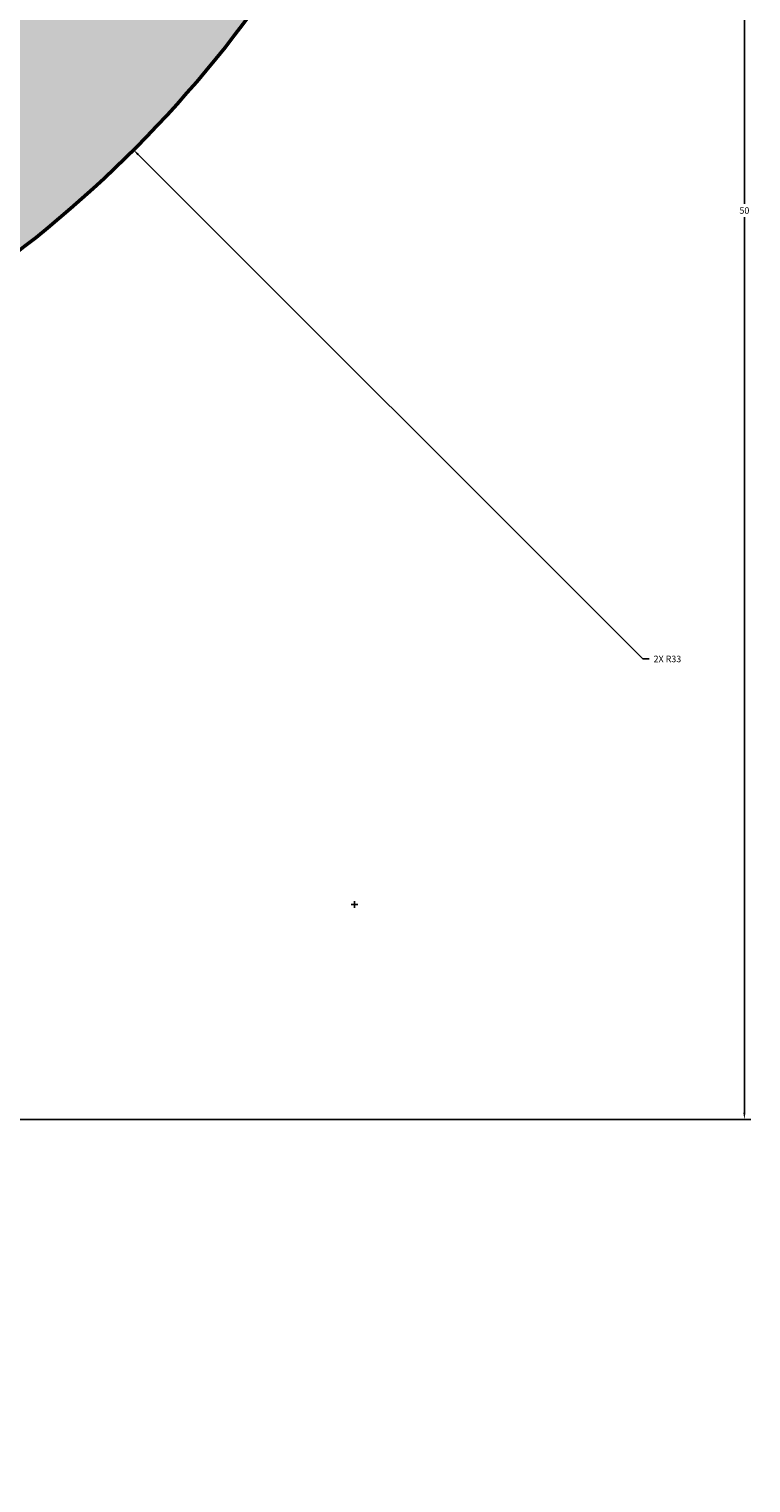
# Model space of a CAD drawing. Units: inches. Extents: x -13 to 107, y -48 to 102.
# Tile 4 of 13: x 48 to 68, y -47 to -7. Entities that reach past the tile are written whole.
import ezdxf

# ---------------------------------------------------------------- set-up
doc = ezdxf.new("R2010")
doc.units = ezdxf.units.IN
doc.header["$MEASUREMENT"] = 0
for name, color, linetype, lineweight in [('M-DIMS', 2, 'Continuous', 18), ('M-HATC', 8, 'Continuous', 18), ('M-OUTL', 7, 'Continuous', 50)]:
    doc.layers.add(name, color=color, linetype=linetype, lineweight=lineweight)
doc.styles.get("Standard").update_dxf_attribs({"font": 'arial.ttf'})
doc.dimstyles.get("Standard").update_dxf_attribs({"dimtxt": 0.18, "dimasz": 0.18, "dimexe": 0.18, "dimexo": 0.0625, "dimgap": 0.09, "dimtad": 0, "dimtih": 1, "dimtoh": 1, "dimdec": 4, "dimzin": 0, "dimdsep": 46, "dimtxsty": 'Standard', "dimcen": 0.09, "dimadec": 0, "dimazin": 0, "dimtfac": 1, "dimtdec": 4, "dimtofl": 0, "dimtmove": 0, "dimatfit": 3, "dimfxl": 1, "dimtolj": 1, "dimtzin": 0, "dimarcsym": 0})

# ---------------------------------------------------------------- blocks, each defined once
blk = doc.blocks.new('*D3')
at = {"layer": 'Defpoints', "color": 0, "transparency": 16777216}
for p in [(27.547, 13.408), (67.679, 13.408), (27.547, -36.592)]:
    blk.add_point(p, dxfattribs=at)
at = {"layer": 'M-DIMS', "color": 0, "lineweight": -2, "transparency": 16777216}
for p, q in [((27.609, 13.408), (67.859, 13.408)), ((67.679, 13.228), (67.679, -11.41)), ((67.679, -36.412), (67.679, -11.774)), ((27.609, -36.592), (67.859, -36.592))]:
    blk.add_line(p, q, dxfattribs=at)
at = {"layer": 'M-DIMS', "color": 0, "transparency": 16777216}
for points in [[(67.649, 13.228), (67.709, 13.228), (67.679, 13.408)], [(67.649, -36.412), (67.709, -36.412), (67.679, -36.592)]]:
    blk.add_solid(points, dxfattribs=at)
at = {"layer": 'M-DIMS', "color": 0, "transparency": 16777216, "insert": (67.679, -11.592), "char_height": 0.18, "attachment_point": 5}
blk.add_mtext('\\A1;50', dxfattribs=at)
blk = doc.blocks.new('*D8')
at = {"layer": 'Defpoints', "color": 0, "transparency": 16777216}
for p in [(27.547, 13.408), (50.882, -9.927)]:
    blk.add_point(p, dxfattribs=at)
at = {"layer": 'M-DIMS', "color": 0, "lineweight": -2, "transparency": 16777216}
for p, q in [((27.457, 13.408), (27.637, 13.408)), ((27.547, 13.318), (27.547, 13.498)), ((64.882, -23.927), (51.009, -10.054)), ((65.062, -23.927), (64.882, -23.927))]:
    blk.add_line(p, q, dxfattribs=at)
at = {"layer": 'M-DIMS', "color": 0, "transparency": 16777216}
blk.add_solid([(51.03, -10.033), (50.988, -10.075), (50.882, -9.927)], dxfattribs=at)
at = {"layer": 'M-DIMS', "color": 0, "transparency": 16777216, "insert": (65.562, -23.927), "char_height": 0.18, "attachment_point": 5}
blk.add_mtext('\\A1;2X R33', dxfattribs=at)
blk = doc.blocks.new('*D11')
at = {"layer": 'Defpoints', "color": 0, "transparency": 16777216}
for p in [(38.592, -22.767), (56.959, -30.682)]:
    blk.add_point(p, dxfattribs=at)
at = {"layer": 'M-DIMS', "color": 0, "lineweight": -2, "transparency": 16777216}
for p, q in [((27.392, -18.018), (27.572, -18.018)), ((27.572, -18.018), (38.427, -22.696)), ((56.869, -30.682), (57.049, -30.682)), ((56.959, -30.772), (56.959, -30.592))]:
    blk.add_line(p, q, dxfattribs=at)
at = {"layer": 'M-DIMS', "color": 0, "transparency": 16777216}
blk.add_solid([(38.438, -22.668), (38.415, -22.724), (38.592, -22.767)], dxfattribs=at)
at = {"layer": 'M-DIMS', "color": 0, "transparency": 16777216, "insert": (26.892, -18.018), "char_height": 0.18, "attachment_point": 5}
blk.add_mtext('\\A1;2X R20', dxfattribs=at)

msp = doc.modelspace()

# ---------------------------------------------------------------- hatches: boundary and pattern name
at = {"layer": 'M-HATC'}
h = msp.add_hatch(color=256, dxfattribs=at)
h.set_gradient(color1=(88, 186, 72), color2=(241, 235, 31), tint=1)
h.paths.add_polyline_path([(45.86, -14.044, 0.420873), (54.577, 32.339, -0.184081), (43.437, 76.537, 1.124637), (11.657, 76.537, -0.184081), (0.517, 32.339, 0.420873), (9.234, -14.044, -0.304084), (17.743, -34.622, 1.220926), (37.351, -34.622, -0.304084)])
h.paths.add_polyline_path([(33.479, -5.692, 0.859727), (21.615, -5.692, -0.111692), (13.972, -1.28, 0.859727), (8.04, 8.995, -0.111692), (8.04, 17.82, 0.859727), (13.972, 28.095, -0.111692), (21.615, 32.508, 0.859727), (33.479, 32.508, -0.111692), (41.122, 28.095, 0.859727), (47.054, 17.82, -0.111692), (47.054, 8.995, 0.859727), (41.122, -1.28, -0.111692)], flags=16)
h.paths.add_polyline_path([(32.547, -36.592, -1), (22.547, -36.592, -1)], flags=16)
h.paths.add_polyline_path([(17.547, 78.408, -1), (37.547, 78.408, -1)], flags=16)

# ---------------------------------------------------------------- linework, layer by layer
at = {"layer": 'M-OUTL'}
msp.add_arc((27.547, 13.408), 33, 303.707, 35.0067, dxfattribs=at)

# ---------------------------------------------------------------- dimensions: what is measured, and where the dimension line sits
at = {"layer": 'M-DIMS'}
for center, mpoint, picture, middle in [((27.547, 13.408), (50.882, -9.927), '*D8', (65.562, -23.927)), ((56.959, -30.682), (38.592, -22.767), '*D11', (26.892, -18.018))]:
    dim = msp.add_radius_dim(center=center, mpoint=mpoint, text='2X <>', dimstyle='Standard', override={"dimdec": 0, "dimlfac": 1, "dimrnd": 0, "dimzin": 0, "dimdsep": 46, "dimlunit": 2}, dxfattribs=at)
    dim.commit()
    dim.dimension.update_dxf_attribs({"geometry": picture, "text_midpoint": middle, "dimtype": 164})
dim = msp.add_linear_dim(base=(67.679, 13.408), p1=(27.547, -36.592), p2=(27.547, 13.408), angle=90, dimstyle='Standard', override={"dimdec": 0, "dimlfac": 1, "dimrnd": 0, "dimzin": 0, "dimdsep": 46, "dimlunit": 2}, dxfattribs=at)
dim.commit()
dim.dimension.update_dxf_attribs({"geometry": '*D3', "text_midpoint": (67.679, -11.592)})

doc.saveas('drawing.dxf')
